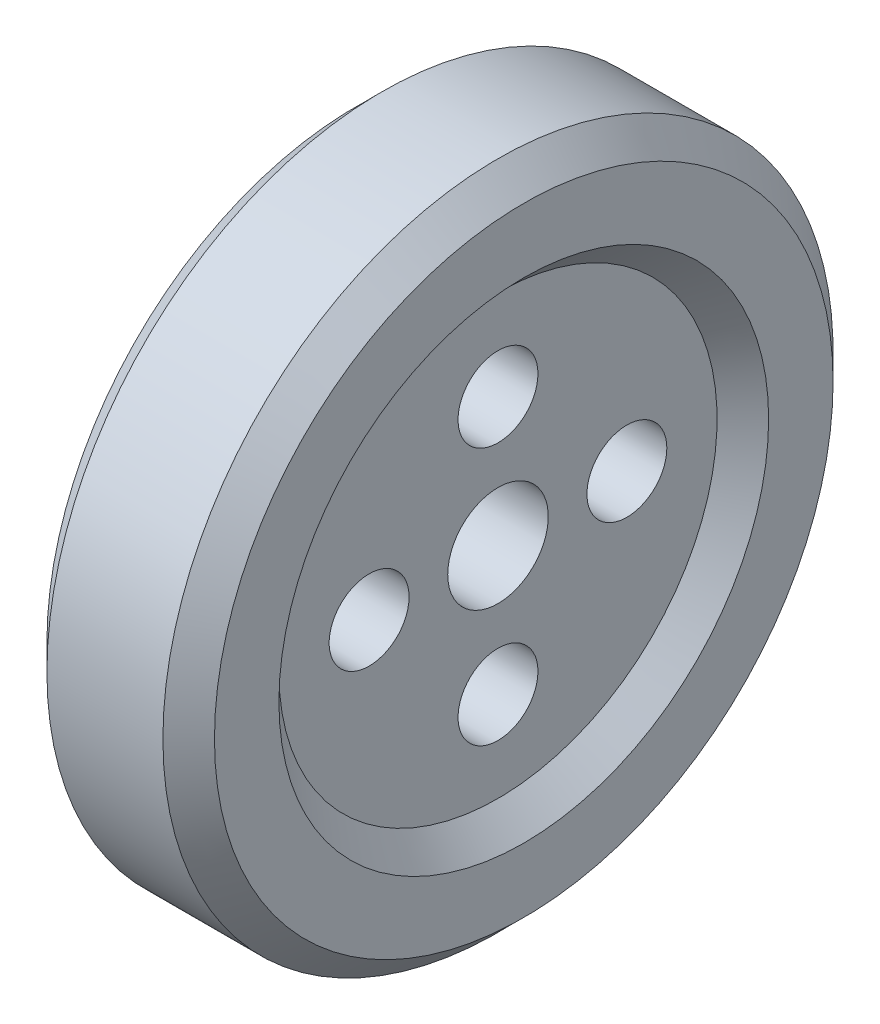
from build123d import *

# Parameters (mm, degrees)
THREAD_HOLES_5X_REACH = 385.797
THREAD_HOLES_SKETCH_R = 31


with BuildPart() as part:
    # Disc Profile Sketch → Button Disc Body (revolve)
    with BuildSketch(Plane.XY, mode=Mode.PRIVATE) as button_disc_body_sk:
        Polygon((-45, 260), (-65, 240), (-65, 190), (-45, 170), (-45, 39), (45, 39), (45, 170), (65, 190), (65, 240), (45, 260), align=None)
    revolve(button_disc_body_sk.sketch.rotate(Axis((-186.115918114, 0, 0), (1, 0, 0)), 90), axis=Axis((-186.115918114, 0, 0), (1, 0, 0)))

    # Thread Holes Sketch → Thread Holes 5x (cut, up to next)
    with BuildSketch(Plane(origin=(45, 0, 0), x_dir=(0, 0, -1), z_dir=(1, 0, 0)), mode=Mode.PRIVATE) as thread_holes_5x_sk1:
        with Locations((0, 100)):
            Circle(THREAD_HOLES_SKETCH_R)
    thread_holes_5x_tool1 = extrude(thread_holes_5x_sk1.sketch, amount=-THREAD_HOLES_5X_REACH, mode=Mode.PRIVATE) & part.part
    # Thread Holes Sketch → Thread Holes 5x (cut, up to next)
    with BuildSketch(Plane(origin=(45, 0, 0), x_dir=(0, 0, -1), z_dir=(1, 0, 0)), mode=Mode.PRIVATE) as thread_holes_5x_sk2:
        with Locations((100, 0)):
            Circle(THREAD_HOLES_SKETCH_R)
    thread_holes_5x_tool2 = extrude(thread_holes_5x_sk2.sketch, amount=-THREAD_HOLES_5X_REACH, mode=Mode.PRIVATE) & part.part
    # Thread Holes Sketch → Thread Holes 5x (cut, up to next)
    with BuildSketch(Plane(origin=(45, 0, 0), x_dir=(0, 0, -1), z_dir=(1, 0, 0)), mode=Mode.PRIVATE) as thread_holes_5x_sk3:
        with Locations((0, -100)):
            Circle(THREAD_HOLES_SKETCH_R)
    thread_holes_5x_tool3 = extrude(thread_holes_5x_sk3.sketch, amount=-THREAD_HOLES_5X_REACH, mode=Mode.PRIVATE) & part.part
    # Thread Holes Sketch → Thread Holes 5x (cut, up to next)
    with BuildSketch(Plane(origin=(45, 0, 0), x_dir=(0, 0, -1), z_dir=(1, 0, 0)), mode=Mode.PRIVATE) as thread_holes_5x_sk4:
        with Locations((-100, 0)):
            Circle(THREAD_HOLES_SKETCH_R)
    thread_holes_5x_tool4 = extrude(thread_holes_5x_sk4.sketch, amount=-THREAD_HOLES_5X_REACH, mode=Mode.PRIVATE) & part.part
    add(thread_holes_5x_tool1.solids().sort_by_distance((45, 100, 0))[0], mode=Mode.SUBTRACT)
    add(thread_holes_5x_tool2.solids().sort_by_distance((45, 0, -100))[0], mode=Mode.SUBTRACT)
    add(thread_holes_5x_tool3.solids().sort_by_distance((45, -100, 0))[0], mode=Mode.SUBTRACT)
    add(thread_holes_5x_tool4.solids().sort_by_distance((45, 0, 100))[0], mode=Mode.SUBTRACT)


solid = part.part
